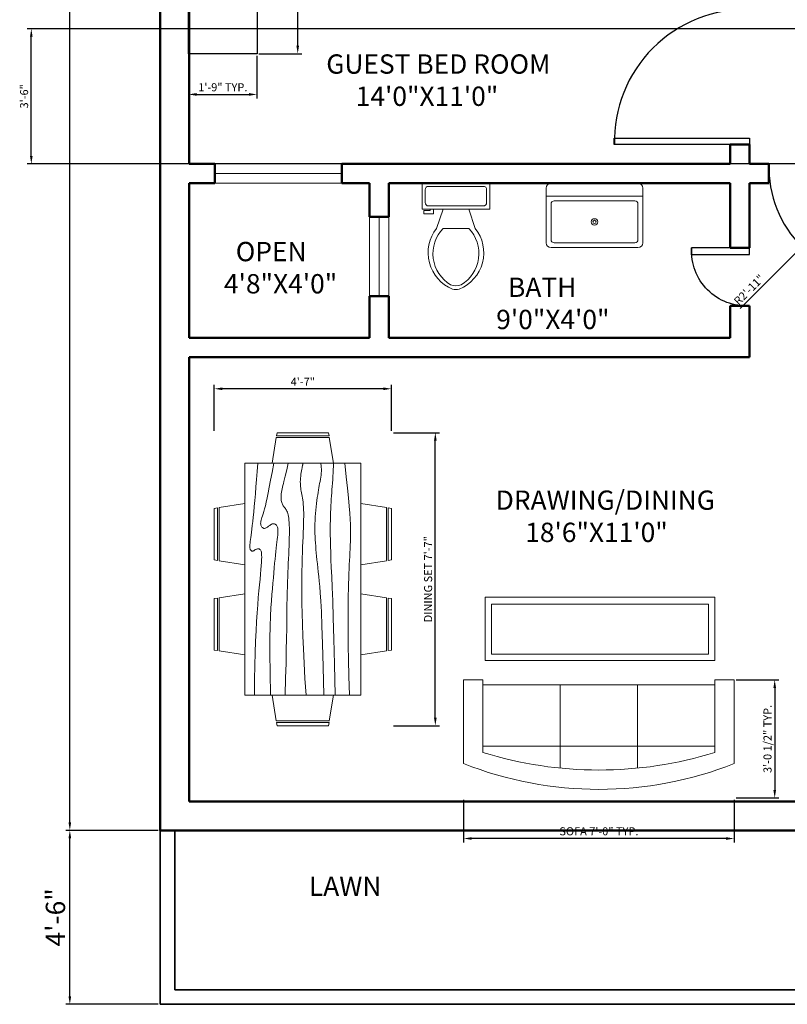
# Model space of a CAD drawing. Units: inches. Extents: x 2690 to 3266, y 1440 to 2261.
# Tile 1 of 4: x 2692 to 2930, y 1484 to 1790. Entities that reach past the tile are written whole.
import ezdxf

# ---------------------------------------------------------------- set-up
doc = ezdxf.new("R2010")
doc.units = ezdxf.units.IN
for name, color, linetype, lineweight in [('A-ANNO-DIMS', 2, 'Continuous', 18), ('A-AREA-IDEN', 7, 'Continuous', 25), ('A-DOOR', 4, 'Continuous', 25), ('A-FLOR-CASE', 9, 'Continuous', 25), ('A-FLOR-FIXT', 9, 'Continuous', 18), ('A-FURN', 8, 'Continuous', 18), ('A-GLAZ', 3, 'Continuous', 18), ('A-WALL', 7, 'Continuous', 50), ('L-SITE-WALL', 7, 'Continuous', 35)]:
    doc.layers.add(name, color=color, linetype=linetype, lineweight=lineweight)
doc.styles.get("Standard").update_dxf_attribs({"font": 'arial.ttf'})
doc.dimstyles.new('ISO-25', dxfattribs={"dimtxt": 2.5, "dimasz": 2.5, "dimexe": 1.25, "dimexo": 0.625, "dimtad": 1, "dimlunit": 3, "dimtxsty": 'Standard', "dimcen": 2.5, "dimadec": 0, "dimazin": 0, "dimtfac": 1, "dimtmove": 0, "dimatfit": 3, "dimfxl": 1, "dimarcsym": 0})

# ---------------------------------------------------------------- blocks, each defined once
blk = doc.blocks.new('Sofa - Roundback 7 ft.')
for p, q in [((-12.00002, -32.4421), (-12.00003, -6.5971)), ((11.99997, -32.4421), (11.99998, -6.5971)), ((-36.000027, -34), (-36.000027, -11.4696)), ((35.99998, -34), (35.99998, -11.4696)), ((-35.999844, -13.3819), (35.9998, -13.3819)), ((-36.000027, -32.4421), (35.99998, -32.4421))]:
    blk.add_line(p, q)
for points in [[(-36.000027, -34), (-42.000027, -34), (-42.000027, -8)], [(41.99998, -8), (41.99998, -34), (35.99998, -34)]]:
    blk.add_lwpolyline(points)
for centre, radius, start, end in [((0, -114.25), 114.25, 68.43141, 111.5686), ((-0.00001, -127.1968), 121.1968, 72.72033, 107.2797)]:
    blk.add_arc(centre, radius, start, end)
blk = doc.blocks.new('Dining Set - 36 x 72 in.')
for p, q in [((-22.2343, 26.00059), (-23.4847, 17.99762)), ((-22.2304, 26), (-5.7608, 26)), ((-22, 27.5), (-22.1562, 26.50042)), ((-5.8416, 26.5), (-22.1534, 26.5)), ((-22, 27.5), (-6, 27.5)), ((-5.8437, 26.49966), (-6, 27.5)), ((-4.5152, 17.99762), (-5.7655, 25.99926)), ((5.7657, 26.00059), (4.5153, 17.99762)), ((5.7696, 26), (22.2392, 26)), ((6, 27.5), (5.8438, 26.50042)), ((22.1584, 26.5), (5.8466, 26.5)), ((6, 27.5), (22, 27.5)), ((22.1563, 26.49966), (22, 27.5)), ((23.4848, 17.99762), (22.2345, 25.99926)), ((36, 18), (-36, 18)), ((-36, 18), (-36, -18)), ((36, -18), (36, 18)), ((-44.0006, 8.23428), (-35.9976, 9.48474)), ((44.0006, 8.23428), (35.9976, 9.48474)), ((-45.5, 8), (-44.5004, 8.15617)), ((-45.5, 8), (-45.5, -8)), ((-44.5, -8.15843), (-44.5, 8.15338)), ((-44, 8.23041), (-44, -8.23915)), ((44, 8.23041), (44, -8.23915)), ((44.5, -8.15843), (44.5, 8.15338)), ((45.5, 8), (44.5005, 8.15617)), ((45.5, 8), (45.5, -8)), ((-44.4997, -8.15631), (-45.5, -8)), ((-35.9976, -9.48476), (-43.9993, -8.2345)), ((35.9976, -9.48476), (43.9993, -8.2345)), ((44.4997, -8.15631), (45.5, -8)), ((-36, -18), (36, -18)), ((-22.2343, -26.0006), (-23.4847, -17.99762)), ((-4.5152, -17.99762), (-5.7655, -25.99928)), ((5.7657, -26.0006), (4.5153, -17.99762)), ((23.4848, -17.99762), (22.2345, -25.99928)), ((-22.2304, -26), (-5.7608, -26)), ((-22, -27.5), (-22.1562, -26.50044)), ((-5.8416, -26.5), (-22.1534, -26.5)), ((-22, -27.5), (-6, -27.5)), ((-5.8437, -26.49967), (-6, -27.5)), ((5.7696, -26), (22.2392, -26)), ((6, -27.5), (5.8438, -26.50044)), ((22.1584, -26.5), (5.8466, -26.5)), ((6, -27.5), (22, -27.5)), ((22.1563, -26.49967), (22, -27.5))]:
    blk.add_line(p, q)
for points in [[(-36, 15), (-31.1772, 14.97754), (-26.8079, 14.91406), (-22.8538, 14.81543), (-19.276, 14.6875), (-16.0362, 14.53613), (-13.0957, 14.36718), (-10.4159, 14.18652), (-7.9583, 14), (-5.6904, 13.81315), (-3.6035, 13.63021), (-1.6954, 13.45508), (0.0365, 13.29166), (1.5945, 13.14388), (2.9811, 13.01562), (4.1988, 12.9108), (5.25, 12.83333), (6.1393, 12.78613), (6.8802, 12.76823), (7.4883, 12.77767), (7.9792, 12.8125), (8.3685, 12.87077), (8.6719, 12.95052), (8.9049, 13.0498), (9.0833, 13.16666), (9.2205, 13.29899), (9.3216, 13.44401), (9.3895, 13.59879), (9.4271, 13.76041), (9.4373, 13.92594), (9.4232, 14.09245), (9.3875, 14.257), (9.3333, 14.41666), (9.2638, 14.56917), (9.1836, 14.71484), (9.0975, 14.85465), (9.0104, 14.98958), (8.9272, 15.1206), (8.8529, 15.2487), (8.7922, 15.37483), (8.75, 15.5), (8.7305, 15.62467), (8.7344, 15.74739), (8.7617, 15.86621), (8.8125, 15.97916), (8.8867, 16.08431), (8.9844, 16.17968), (9.1055, 16.26334), (9.25, 16.33333), (9.4189, 16.38802), (9.6172, 16.42708), (9.8506, 16.45052), (10.125, 16.45833), (10.4463, 16.45052), (10.8203, 16.42708), (11.2529, 16.38802), (11.75, 16.33333), (12.3184, 16.26318), (12.9694, 16.17838), (13.7151, 16.07991), (14.5677, 15.96875), (15.5395, 15.84586), (16.6426, 15.71224), (17.8893, 15.56884), (19.2917, 15.41666), (20.859, 15.25667), (22.5879, 15.08984), (24.4721, 14.91715), (26.5052, 14.73958), (28.6809, 14.5581), (30.9929, 14.3737), (33.4347, 14.18733), (36, 14)], [(-36, 10), (-28.9766, 10.14274), (-23.1725, 10.20442), (-18.4241, 10.19775), (-14.5677, 10.13541), (-11.4399, 10.03011), (-8.877, 9.89453), (-6.7154, 9.74137), (-4.7917, 9.58333), (-2.9698, 9.43082), (-1.2246, 9.28515), (0.4415, 9.14534), (2.026, 9.01041), (3.5266, 8.87939), (4.9408, 8.7513), (6.266, 8.62516), (7.5, 8.5), (8.6411, 8.37549), (9.6914, 8.2539), (10.6538, 8.13818), (11.5312, 8.03125), (12.3267, 7.93603), (13.043, 7.85547), (13.6831, 7.79248), (14.25, 7.75), (14.7471, 7.7303), (15.1797, 7.73307), (15.5537, 7.75732), (15.875, 7.80208), (16.1494, 7.86637), (16.3828, 7.94922), (16.5811, 8.04964), (16.75, 8.16666), (16.8944, 8.29915), (17.0143, 8.44531), (17.1089, 8.60319), (17.1771, 8.77083), (17.218, 8.94629), (17.2305, 9.1276), (17.2137, 9.31282), (17.1667, 9.5), (17.0895, 9.6875), (16.987, 9.875), (16.8649, 10.0625), (16.7292, 10.25), (16.5856, 10.4375), (16.4401, 10.625), (16.2985, 10.8125), (16.1667, 11), (16.05, 11.18733), (15.9518, 11.3737), (15.8752, 11.5581), (15.8229, 11.73958), (15.798, 11.91715), (15.8034, 12.08984), (15.842, 12.25667), (15.9167, 12.41666), (16.0295, 12.56836), (16.1784, 12.70833), (16.3605, 12.83268), (16.5729, 12.9375), (16.8127, 13.01888), (17.0768, 13.07291), (17.3625, 13.0957), (17.6667, 13.08333), (17.9894, 13.03312), (18.3418, 12.94726), (18.7382, 12.82918), (19.1927, 12.68229), (19.7195, 12.51001), (20.3327, 12.31575), (21.0465, 12.10294), (21.875, 11.875), (22.8357, 11.63354), (23.959, 11.37304), (25.2786, 11.08618), (26.8282, 10.76562), (28.6414, 10.40405), (30.752, 9.99414), (33.1936, 9.52856), (36, 9)], [(-36, 5.5), (-30.7157, 5.3348), (-26.069, 5.20963), (-21.9946, 5.11767), (-18.4271, 5.05208), (-15.3009, 5.00602), (-12.5508, 4.97265), (-10.1112, 4.94515), (-7.9167, 4.91666), (-5.909, 4.88167), (-4.0586, 4.83984), (-2.3429, 4.79215), (-0.7396, 4.73958), (0.7739, 4.6831), (2.22, 4.6237), (3.6213, 4.56233), (5, 4.5), (6.373, 4.43782), (7.7344, 4.3776), (9.0723, 4.32129), (10.375, 4.27083), (11.6309, 4.22819), (12.8281, 4.19531), (13.9551, 4.17415), (15, 4.16666), (15.954, 4.17448), (16.819, 4.19791), (17.6001, 4.23698), (18.3021, 4.29166), (18.9299, 4.36198), (19.4883, 4.44791), (19.9823, 4.54948), (20.4167, 4.66666), (20.7969, 4.79899), (21.1302, 4.94401), (21.4245, 5.09879), (21.6875, 5.26041), (21.9271, 5.42594), (22.1511, 5.59245), (22.3672, 5.757), (22.5834, 5.91666), (22.8065, 6.06868), (23.0404, 6.21093), (23.2879, 6.34147), (23.5521, 6.45833), (23.8358, 6.55957), (24.142, 6.64323), (24.4735, 6.70735), (24.8334, 6.75), (25.2235, 6.76969), (25.642, 6.76692), (26.0858, 6.74267), (26.5521, 6.69791), (27.0379, 6.63362), (27.5404, 6.55078), (28.0565, 6.45036), (28.5834, 6.33333), (29.1242, 6.19987), (29.7071, 6.04687), (30.3661, 5.87044), (31.1354, 5.66666), (32.0493, 5.43164), (33.142, 5.16146), (34.4475, 4.85221), (36, 4.5)], [(-36, -1), (-30.7915, -0.6591), (-26.0195, -0.38216), (-21.6519, -0.16284), (-17.6563, 0.00521), (-14.0005, 0.12833), (-10.6523, 0.21289), (-7.5796, 0.26522), (-4.75, 0.29166), (-2.134, 0.29793), (0.2878, 0.28711), (2.5317, 0.26163), (4.6146, 0.22396), (6.5529, 0.17651), (8.3633, 0.12174), (10.0623, 0.06209), (11.6667, 0), (13.1899, -0.06201), (14.6341, -0.1211), (15.9982, -0.17432), (17.2813, -0.21875), (18.4823, -0.25147), (19.6003, -0.26953), (20.6343, -0.27002), (21.5834, -0.25), (22.4481, -0.20768), (23.2357, -0.14584), (23.9549, -0.06836), (24.6146, 0.02083), (25.2235, 0.11784), (25.7904, 0.21875), (26.3241, 0.31966), (26.8334, 0.41666), (27.3265, 0.50618), (27.8099, 0.58593), (28.2894, 0.65397), (28.7709, 0.70833), (29.2601, 0.74707), (29.763, 0.76823), (30.2855, 0.76985), (30.8334, 0.75), (31.4088, 0.70784), (31.9994, 0.64713), (32.589, 0.57275), (33.1615, 0.48958), (33.7008, 0.4025), (34.1908, 0.3164), (34.6153, 0.23616), (34.9584, 0.16666), (35.2099, 0.11165), (35.3848, 0.07031), (35.504, 0.04069), (35.5886, 0.02083), (35.6594, 0.00879), (35.7377, 0.0026), (35.8442, 0.00032), (36, 0)], [(-36, -6.5), (-27.1843, -6.31267), (-20.084, -6.1263), (-14.469, -5.9419), (-10.1094, -5.76042), (-6.7752, -5.58285), (-4.2363, -5.41016), (-2.2629, -5.24333), (-0.625, -5.08334), (0.8708, -4.93099), (2.2715, -4.78646), (3.5872, -4.64974), (4.8281, -4.52084), (6.0046, -4.39974), (7.127, -4.28646), (8.2053, -4.18099), (9.25, -4.08334), (10.2705, -3.99382), (11.2734, -3.91407), (12.2647, -3.84603), (13.25, -3.79167), (14.2354, -3.75293), (15.2266, -3.73177), (16.2295, -3.73015), (17.25, -3.75), (18.2912, -3.79248), (19.3451, -3.85547), (20.4009, -3.93604), (21.4479, -4.03125), (22.4754, -4.13819), (23.4727, -4.25391), (24.4289, -4.37549), (25.3334, -4.5), (26.1785, -4.62492), (26.9694, -4.74935), (27.7145, -4.87281), (28.4219, -4.99479), (29.1, -5.11483), (29.7572, -5.23242), (30.4016, -5.34709), (31.0417, -5.45834), (31.6837, -5.56437), (32.3262, -5.65821), (32.9658, -5.73153), (33.599, -5.77604), (34.2224, -5.78345), (34.8327, -5.74545), (35.4264, -5.65373), (36, -5.5)], [(-36, -10), (-26.4022, -9.81299), (-18.4675, -9.62891), (-11.9839, -9.45069), (-6.7396, -9.28125), (-2.5226, -9.12354), (0.8789, -8.98047), (3.6769, -8.85498), (6.0833, -8.75), (8.2767, -8.66765), (10.3021, -8.60677), (12.1712, -8.56543), (13.8958, -8.54167), (15.4876, -8.53353), (16.9583, -8.53907), (18.3197, -8.55632), (19.5834, -8.58334), (20.7616, -8.61841), (21.8685, -8.66081), (22.9188, -8.71004), (23.9271, -8.76563), (24.9081, -8.82707), (25.8763, -8.89388), (26.8465, -8.96558), (27.8334, -9.04167), (28.8474, -9.12118), (29.8828, -9.20117), (30.93, -9.27824), (31.9792, -9.34896), (33.0205, -9.40991), (34.0443, -9.45768), (35.0407, -9.48885), (36, -9.5)], [(-36, -14.5), (-30.0881, -14.33513), (-25.0332, -14.21224), (-20.7312, -14.12647), (-17.0781, -14.07292), (-13.97, -14.04671), (-11.3027, -14.04297), (-8.9724, -14.05681), (-6.875, -14.08334), (-4.9224, -14.11833), (-3.0905, -14.16016), (-1.3709, -14.20785), (0.2448, -14.26042), (1.7647, -14.3169), (3.1973, -14.3763), (4.5507, -14.43767), (5.8333, -14.5), (7.0554, -14.5621), (8.235, -14.62175), (9.3922, -14.67652), (10.5469, -14.72396), (11.7192, -14.76164), (12.929, -14.78711), (14.1965, -14.79794), (15.5417, -14.79167), (16.9933, -14.76424), (18.6152, -14.70508), (20.4804, -14.60197), (22.6615, -14.44271), (25.2312, -14.21509), (28.2624, -13.9069), (31.8277, -13.50594), (36, -13)]]:
    blk.add_lwpolyline(points)
blk = doc.blocks.new('Toilet - top')
for p, q in [((9.5, -6), (9.5, -2)), ((-10, -8.5), (-8, -8.5)), ((-10, -9.5), (-10, -8.5)), ((-8, -8.5), (-8, -8)), ((-7, -8), (-7, -9.5)), ((-4, -8), (-6, -14)), ((4, -8), (6, -14)), ((-7, -9.5), (-10, -9.5)), ((4, -14), (-4, -14))]:
    blk.add_line(p, q)
blk.add_lwpolyline([(10.5, -8), (10.5, 0), (-10.5, 0), (-10.5, -8)], close=True)
for points in [[(-9.5, -2), (-9.5, -6)], [(8.5, -1), (-8.5, -1)], [(-8.5, -7), (8.5, -7)]]:
    blk.add_lwpolyline(points)
for centre, radius, start, end in [((-8.62, -1.88), 0.884, 81.8699, 188.1301), ((8.62, -1.88), 0.884, 351.8699, 98.1301), ((-8.62, -6.12), 0.884, 171.8699, 278.1301), ((8.62, -6.12), 0.884, 261.8699, 8.1301), ((3.52, -21.58), 12.17, 141.4691, 247.9714), ((4.2, -21.82), 11.33, 136.3677, 238.9468), ((-3.52, -21.58), 12.17, 292.0284, 38.5307), ((-4.2, -21.82), 11.33, 301.053, 43.6321), ((0, -27.88), 4, 245.7318, 294.2682), ((0, -29), 4, 254.8605, 285.1395)]:
    blk.add_arc(centre, radius, start, end)
blk = doc.blocks.new('Sink-single - 30 in top')
blk.add_line((-15, -3.999996), (15, -3.999996))
for points in [[(-13.5, 0), (13.5, 0)], [(-15, -18.499996), (-15, -1.5)], [(15, -1.5), (15, -18.499996)], [(-12.5, -5.499996), (12.5, -5.499996)], [(-13.5, -17.499996), (-13.5, -6.499996)], [(13.5, -6.499996), (13.5, -17.499996)], [(13.5, -19.999996), (-13.5, -19.999996)], [(12.5, -18.499996), (-12.5, -18.499996)]]:
    blk.add_lwpolyline(points)
for radius in [1, 0.5]:
    blk.add_circle((0, -11.999996), radius)
for centre, radius, start, end in [((-13.5, -1.5), 1.5, 90, 180), ((13.5, -1.5), 1.5, 0, 90), ((-12.5, -6.499996), 1, 90, 180), ((12.5, -6.499996), 1, 0, 90), ((-12.5, -17.499996), 1, 180, 270), ((12.5, -17.499996), 1, 270, 0), ((-13.5, -18.499996), 1.5, 180, 270), ((13.5, -18.499996), 1.5, 270, 0)]:
    blk.add_arc(centre, radius, start, end)
blk = doc.blocks.new('*D13')
at = {"layer": 'A-ANNO-DIMS', "color": 0, "lineweight": -2, "transparency": 16777216}
for p, q in [((2734.85, 2204.49), (2706.14, 2204.49)), ((2707.39, 1540.99), (2707.39, 2201.99)), ((2734.85, 1538.49), (2706.14, 1538.49))]:
    blk.add_line(p, q, dxfattribs=at)
at = {"layer": 'A-ANNO-DIMS', "color": 0, "transparency": 16777216}
for points in [[(2706.97, 2201.99), (2707.81, 2201.99), (2707.39, 2204.49)], [(2706.97, 1540.99), (2707.81, 1540.99), (2707.39, 1538.49)]]:
    blk.add_solid(points, dxfattribs=at)
at = {"layer": 'Defpoints', "color": 0, "transparency": 16777216}
for p in [(2707.39, 2204.49), (2735.48, 2204.49), (2735.48, 1538.49)]:
    blk.add_point(p, dxfattribs=at)
at = {"layer": 'A-ANNO-DIMS', "color": 0, "transparency": 16777216, "insert": (2703.7, 1871.49), "char_height": 6, "attachment_point": 5, "rotation": 90}
blk.add_mtext('55\'-6"', dxfattribs=at)
blk = doc.blocks.new('*D14')
at = {"layer": 'A-ANNO-DIMS', "color": 0, "lineweight": -2, "transparency": 16777216}
for p, q in [((2734.85, 1538.49), (2706.14, 1538.49)), ((2707.39, 1486.99), (2707.39, 1535.99)), ((2734.85, 1484.49), (2706.14, 1484.49))]:
    blk.add_line(p, q, dxfattribs=at)
at = {"layer": 'A-ANNO-DIMS', "color": 0, "transparency": 16777216}
for points in [[(2706.97, 1535.99), (2707.81, 1535.99), (2707.39, 1538.49)], [(2706.97, 1486.99), (2707.81, 1486.99), (2707.39, 1484.49)]]:
    blk.add_solid(points, dxfattribs=at)
at = {"layer": 'Defpoints', "color": 0, "transparency": 16777216}
for p in [(2707.39, 1538.49), (2735.48, 1538.49), (2735.48, 1484.49)]:
    blk.add_point(p, dxfattribs=at)
at = {"layer": 'A-ANNO-DIMS', "color": 0, "transparency": 16777216, "insert": (2703.7, 1511.49), "char_height": 6, "attachment_point": 5, "rotation": 90}
blk.add_mtext('4\'-6"', dxfattribs=at)
blk = doc.blocks.new('DOOR-SWING-18IN')
for p, q in [((0, 0), (0, 18)), ((0, 18), (2, 18)), ((2, 18), (2, 0)), ((2, 0), (0, 0))]:
    blk.add_line(p, q)
blk.add_arc((1, 1), 17.03, 356.6335, 93.3665)
blk = doc.blocks.new('DOOR-SWING-42IN')
for p, q in [((-42, 0), (-42, 2)), ((-42, 2), (0, 2)), ((0, 0), (-42, 0)), ((0, 2), (0, 0))]:
    blk.add_line(p, q)
blk.add_arc((-1, 1), 41.01, 88.6028, 181.3972)
blk = doc.blocks.new('WARDROBE-PLAN')
blk.add_lwpolyline([(0, 0), (21.23, 0), (21.23, -84.36), (0, -84.36)], close=True)
blk = doc.blocks.new('*D31')
at = {"layer": 'A-ANNO-DIMS', "color": 0, "lineweight": -2, "transparency": 16777216}
for p, q in [((2766.13, 1864.09), (2779.41, 1864.09)), ((2778.16, 1782.23), (2778.16, 1861.59)), ((2766.13, 1779.73), (2779.41, 1779.73))]:
    blk.add_line(p, q, dxfattribs=at)
at = {"layer": 'A-ANNO-DIMS', "color": 0, "transparency": 16777216}
for points in [[(2777.74, 1861.59), (2778.58, 1861.59), (2778.16, 1864.09)], [(2777.74, 1782.23), (2778.58, 1782.23), (2778.16, 1779.73)]]:
    blk.add_solid(points, dxfattribs=at)
at = {"layer": 'Defpoints', "color": 0, "transparency": 16777216}
for p in [(2765.51, 1864.09), (2778.16, 1864.09), (2765.51, 1779.73)]:
    blk.add_point(p, dxfattribs=at)
at = {"layer": 'A-ANNO-DIMS', "color": 0, "transparency": 16777216, "insert": (2776.24, 1821.91), "char_height": 2.5, "attachment_point": 5, "rotation": 90}
blk.add_mtext('WARDROBE 7\'-0 1/2" TYP.', dxfattribs=at)
blk = doc.blocks.new('*D32')
at = {"layer": 'A-ANNO-DIMS', "color": 0, "lineweight": -2, "transparency": 16777216}
for p, q in [((2744.28, 1779.11), (2744.28, 1765.83)), ((2765.51, 1779.11), (2765.51, 1765.83)), ((2746.78, 1767.08), (2763.01, 1767.08))]:
    blk.add_line(p, q, dxfattribs=at)
at = {"layer": 'A-ANNO-DIMS', "color": 0, "transparency": 16777216}
for points in [[(2746.78, 1767.5), (2746.78, 1766.66), (2744.28, 1767.08)], [(2763.01, 1767.5), (2763.01, 1766.66), (2765.51, 1767.08)]]:
    blk.add_solid(points, dxfattribs=at)
at = {"layer": 'Defpoints', "color": 0, "transparency": 16777216}
for p in [(2744.28, 1779.73), (2765.51, 1779.73), (2765.51, 1767.08)]:
    blk.add_point(p, dxfattribs=at)
at = {"layer": 'A-ANNO-DIMS', "color": 0, "transparency": 16777216, "insert": (2754.9, 1768.98), "char_height": 2.5, "attachment_point": 5}
blk.add_mtext('1\'-9" TYP.', dxfattribs=at)
blk = doc.blocks.new('*D33')
at = {"layer": 'A-ANNO-DIMS', "color": 0, "lineweight": -2, "transparency": 16777216}
for p, q in [((2829.68, 1547.95), (2829.68, 1534.73)), ((2913.68, 1547.95), (2913.68, 1534.73)), ((2911.18, 1535.98), (2832.18, 1535.98))]:
    blk.add_line(p, q, dxfattribs=at)
at = {"layer": 'A-ANNO-DIMS', "color": 0, "transparency": 16777216}
for points in [[(2832.18, 1536.4), (2832.18, 1535.56), (2829.68, 1535.98)], [(2911.18, 1536.4), (2911.18, 1535.56), (2913.68, 1535.98)]]:
    blk.add_solid(points, dxfattribs=at)
at = {"layer": 'Defpoints', "color": 0, "transparency": 16777216}
for p in [(2829.68, 1548.58), (2913.68, 1548.58), (2829.68, 1535.98)]:
    blk.add_point(p, dxfattribs=at)
at = {"layer": 'A-ANNO-DIMS', "color": 0, "transparency": 16777216, "insert": (2871.68, 1537.9), "char_height": 2.5, "attachment_point": 5}
blk.add_mtext('SOFA 7\'-0" TYP.', dxfattribs=at)
blk = doc.blocks.new('*D34')
at = {"layer": 'A-ANNO-DIMS', "color": 0, "lineweight": -2, "transparency": 16777216}
for p, q in [((2914.31, 1585.25), (2927.53, 1585.25)), ((2926.28, 1582.75), (2926.28, 1551.08)), ((2914.31, 1548.58), (2927.53, 1548.58))]:
    blk.add_line(p, q, dxfattribs=at)
at = {"layer": 'A-ANNO-DIMS', "color": 0, "transparency": 16777216}
for points in [[(2925.87, 1582.75), (2926.7, 1582.75), (2926.28, 1585.25)], [(2925.87, 1551.08), (2926.7, 1551.08), (2926.28, 1548.58)]]:
    blk.add_solid(points, dxfattribs=at)
at = {"layer": 'Defpoints', "color": 0, "transparency": 16777216}
for p in [(2913.68, 1585.25), (2913.68, 1548.58), (2926.28, 1548.58)]:
    blk.add_point(p, dxfattribs=at)
at = {"layer": 'A-ANNO-DIMS', "color": 0, "transparency": 16777216, "insert": (2924.37, 1566.91), "char_height": 2.5, "attachment_point": 5, "rotation": 90}
blk.add_mtext('3\'-0 1/2" TYP.', dxfattribs=at)
blk = doc.blocks.new('*D41')
at = {"layer": 'A-ANNO-DIMS', "color": 0, "lineweight": -2, "transparency": 16777216}
for p, q in [((2807.86, 1662.01), (2822.14, 1662.01)), ((2820.89, 1573.51), (2820.89, 1659.51)), ((2807.86, 1571.01), (2822.14, 1571.01))]:
    blk.add_line(p, q, dxfattribs=at)
at = {"layer": 'A-ANNO-DIMS', "color": 0, "transparency": 16777216}
for points in [[(2820.47, 1659.51), (2821.31, 1659.51), (2820.89, 1662.01)], [(2820.47, 1573.51), (2821.31, 1573.51), (2820.89, 1571.01)]]:
    blk.add_solid(points, dxfattribs=at)
at = {"layer": 'Defpoints', "color": 0, "transparency": 16777216}
for p in [(2807.24, 1662.01), (2820.89, 1662.01), (2807.24, 1571.01)]:
    blk.add_point(p, dxfattribs=at)
at = {"layer": 'A-ANNO-DIMS', "color": 0, "transparency": 16777216, "insert": (2818.97, 1616.51), "char_height": 2.5, "attachment_point": 5, "rotation": 90}
blk.add_mtext('DINING SET 7\'-7"', dxfattribs=at)
blk = doc.blocks.new('*D42')
at = {"layer": 'A-ANNO-DIMS', "color": 0, "lineweight": -2, "transparency": 16777216}
for p, q in [((2752.24, 1662.63), (2752.24, 1676.91)), ((2807.24, 1662.63), (2807.24, 1676.91)), ((2804.74, 1675.66), (2754.74, 1675.66))]:
    blk.add_line(p, q, dxfattribs=at)
at = {"layer": 'A-ANNO-DIMS', "color": 0, "transparency": 16777216}
for points in [[(2754.74, 1676.07), (2754.74, 1675.24), (2752.24, 1675.66)], [(2804.74, 1676.07), (2804.74, 1675.24), (2807.24, 1675.66)]]:
    blk.add_solid(points, dxfattribs=at)
at = {"layer": 'Defpoints', "color": 0, "transparency": 16777216}
for p in [(2752.24, 1675.66), (2752.24, 1662.01), (2807.24, 1662.01)]:
    blk.add_point(p, dxfattribs=at)
at = {"layer": 'A-ANNO-DIMS', "color": 0, "transparency": 16777216, "insert": (2779.74, 1677.53), "char_height": 2.5, "attachment_point": 5}
blk.add_mtext('4\'-7"', dxfattribs=at)
blk = doc.blocks.new('*D53')
at = {"layer": 'A-ANNO-DIMS', "color": 0, "lineweight": -2, "transparency": 16777216}
for p, q in [((3073.85, 1787.49), (2694.18, 1787.49)), ((2695.43, 1747.99), (2695.43, 1784.99)), ((3073.85, 1745.49), (2694.18, 1745.49))]:
    blk.add_line(p, q, dxfattribs=at)
at = {"layer": 'A-ANNO-DIMS', "color": 0, "transparency": 16777216}
for points in [[(2695.01, 1784.99), (2695.84, 1784.99), (2695.43, 1787.49)], [(2695.01, 1747.99), (2695.84, 1747.99), (2695.43, 1745.49)]]:
    blk.add_solid(points, dxfattribs=at)
at = {"layer": 'Defpoints', "color": 0, "transparency": 16777216}
for p in [(2695.43, 1787.49), (3074.48, 1787.49), (3074.48, 1745.49)]:
    blk.add_point(p, dxfattribs=at)
at = {"layer": 'A-ANNO-DIMS', "color": 0, "transparency": 16777216, "insert": (2693.52, 1766.49), "char_height": 2.5, "attachment_point": 5, "rotation": 90}
blk.add_mtext('3\'-6"', dxfattribs=at)
blk = doc.blocks.new('*D61')
at = {"layer": 'A-ANNO-DIMS', "color": 0, "lineweight": -2, "transparency": 16777216}
for p, q in [((2959.48, 1744.49), (2934.72, 1719.73)), ((2915.54, 1700.55), (2932.95, 1717.96))]:
    blk.add_line(p, q, dxfattribs=at)
at = {"layer": 'A-ANNO-DIMS', "color": 0, "transparency": 16777216}
blk.add_solid([(2932.65, 1718.25), (2933.24, 1717.66), (2934.72, 1719.73)], dxfattribs=at)
at = {"layer": 'Defpoints', "color": 0, "transparency": 16777216}
for p in [(2959.48, 1744.49), (2934.72, 1719.73)]:
    blk.add_point(p, dxfattribs=at)
at = {"layer": 'A-ANNO-DIMS', "color": 0, "transparency": 16777216, "insert": (2918.53, 1706.2), "char_height": 2.5, "attachment_point": 5, "rotation": 44.9992}
blk.add_mtext('R2\'-11"', dxfattribs=at)

msp = doc.modelspace()

# ---------------------------------------------------------------- linework, layer by layer
at = {"layer": 'A-DOOR'}
msp.add_line((2918.476, 1751.486), (2918.476, 1751.486), dxfattribs=at)
msp.add_arc((2959.476, 1744.486), 35.014, 178.36342, 271.63658, dxfattribs=at)
at = {"layer": 'A-FURN'}
for points in [[(2836.32, 1610.936), (2907.685, 1610.936), (2907.685, 1591.299), (2836.32, 1591.299)], [(2838.284, 1608.799), (2905.73, 1608.799), (2905.73, 1593.248), (2838.284, 1593.248)]]:
    msp.add_lwpolyline(points, close=True, dxfattribs=at)
at = {"layer": 'A-GLAZ'}
for p, q in [((2752.427, 1745.486), (2791.813, 1745.486)), ((2791.813, 1745.486), (2791.813, 1742.486)), ((2791.813, 1742.486), (2752.427, 1742.486)), ((2752.427, 1742.486), (2752.427, 1739.486)), ((2752.427, 1739.486), (2791.813, 1739.486)), ((2800.476, 1729.052), (2800.476, 1704.39)), ((2803.476, 1704.39), (2803.476, 1729.052)), ((2803.476, 1729.052), (2806.476, 1729.052)), ((2806.476, 1729.052), (2806.476, 1704.39)), ((2800.476, 1704.39), (2803.476, 1704.39))]:
    msp.add_line(p, q, dxfattribs=at)
at = {"layer": 'A-WALL'}
for p, q in [((2735.476, 1538.486), (2735.476, 2204.486)), ((2744.476, 1745.486), (2744.476, 1877.486)), ((2912.476, 1745.486), (2912.476, 1751.486)), ((2918.476, 1751.486), (2912.476, 1751.486)), ((2918.476, 1745.486), (2918.476, 1751.486)), ((2918.476, 1745.486), (2918.476, 1751.486)), ((2744.476, 1745.486), (2752.427, 1745.486)), ((2752.427, 1745.486), (2752.427, 1739.486)), ((2791.813, 1745.486), (2791.813, 1739.486)), ((2791.813, 1745.486), (2912.476, 1745.486)), ((2924.476, 1745.486), (2918.476, 1745.486)), ((2924.476, 1739.486), (2924.476, 1745.486)), ((2744.476, 1739.486), (2752.427, 1739.486)), ((2744.476, 1691.486), (2744.476, 1739.486)), ((2791.813, 1739.486), (2800.476, 1739.486)), ((2800.476, 1729.052), (2800.476, 1739.486)), ((2806.476, 1739.486), (2912.476, 1739.486)), ((2806.476, 1729.052), (2806.476, 1739.486)), ((2912.476, 1719.41), (2912.476, 1739.486)), ((2918.476, 1739.486), (2924.476, 1739.486)), ((2918.476, 1719.41), (2918.476, 1739.486)), ((2800.476, 1729.052), (2806.476, 1729.052)), ((2912.476, 1719.41), (2918.476, 1719.41)), ((2800.476, 1691.486), (2800.476, 1704.39)), ((2800.476, 1704.39), (2806.476, 1704.39)), ((2806.476, 1691.486), (2806.476, 1704.39)), ((2912.476, 1691.486), (2912.476, 1701.41)), ((2912.476, 1701.41), (2918.476, 1701.41)), ((2918.476, 1685.486), (2918.476, 1701.41)), ((2744.476, 1691.486), (2800.476, 1691.486)), ((2806.476, 1691.486), (2912.476, 1691.486)), ((2744.476, 1547.486), (2744.476, 1685.486)), ((2744.476, 1685.486), (2918.476, 1685.486)), ((2966.476, 1547.486), (2744.476, 1547.486)), ((2972.476, 1538.486), (2735.476, 1538.486))]:
    msp.add_line(p, q, dxfattribs=at)
at = {"layer": 'L-SITE-WALL'}
for p, q in [((2735.476, 1538.486), (2735.476, 1484.486)), ((2739.976, 1538.486), (2739.976, 1488.986)), ((2739.976, 1488.986), (2989.13, 1488.986)), ((2735.476, 1484.486), (2989.13, 1484.486))]:
    msp.add_line(p, q, dxfattribs=at)

# ---------------------------------------------------------------- block references
at = {"layer": 'A-DOOR'}
msp.add_blockref('DOOR-SWING-42IN', (2918.476, 1751.486), dxfattribs=at)
at = {"layer": 'A-DOOR', "extrusion": (0, 0, -1), "zscale": -1, "rotation": 270.000000000001}
msp.add_blockref('DOOR-SWING-18IN', (-2918.476, 1719.41), dxfattribs=at)
at = {"layer": 'A-FLOR-CASE'}
msp.add_blockref('WARDROBE-PLAN', (2744.283, 1864.093), dxfattribs=at)
at = {"layer": 'A-FLOR-FIXT'}
for name, p in [('Toilet - top', (2827.281, 1739.486)), ('Sink-single - 30 in top', (2870.327, 1739.486))]:
    msp.add_blockref(name, p, dxfattribs=at)
at = {"layer": 'A-FURN'}
for name, p, rotation in [('Dining Set - 36 x 72 in.', (2779.739, 1616.507), 90), ('Sofa - Roundback 7 ft.', (2871.685, 1551.245), 180)]:
    msp.add_blockref(name, p, dxfattribs=dict(at, rotation=rotation))

# ---------------------------------------------------------------- texts
at = {"layer": 'A-AREA-IDEN', "char_height": 6, "attachment_point": 1}
for s, width, heights, insert in [('     GUEST BED ROOM\\P          14\'0"X11\'0"', 101.41733, [40.167], (2777.848, 1779.519)), ('     OPEN\\P   4\'8"X4\'0"', 77.52183, [0], (2749.753, 1721.272)), ('  BATH\\P9\'0"X4\'0"', 77.52183, [0], (2839.799, 1710.186)), ('DRAWING/DINING\\P     18\'6"X11\'0"', 77.52183, [0], (2839.644, 1644.065)), ('   LAWN', 77.52183, [0], (2776.129, 1524.157))]:
    msp.add_mtext_dynamic_manual_height_columns(s, width=width, gutter_width=12.5, heights=heights, dxfattribs=dict(at, insert=insert))

# ---------------------------------------------------------------- dimensions: what is measured, and where the dimension line sits
at = {"layer": 'A-ANNO-DIMS'}
for base, p1, p2, angle, override, picture, middle in [((2707.39, 2204.486), (2735.476, 1538.486), (2735.476, 2204.486), 90, {"dimtxt": 6, "dimclrd": 0, "dimclre": 0, "dimclrt": 0}, '*D13', (2703.701, 1871.486)), ((2695.426, 1787.486), (3074.476, 1745.486), (3074.476, 1787.486), 90, {"dimdec": 1, "dimlfac": 1, "dimrnd": 0, "dimzin": 1, "dimdsep": 46, "dimlunit": 4, "dimfrac": 2}, '*D53', (2693.524, 1766.486)), ((2752.239, 1675.657), (2807.239, 1662.007), (2752.239, 1662.007), 180, {"dimdec": 1, "dimlfac": 1, "dimrnd": 0, "dimzin": 1, "dimdsep": 46, "dimlunit": 4, "dimfrac": 2}, '*D42', (2779.739, 1677.532)), ((2707.39, 1538.486), (2735.476, 1484.486), (2735.476, 1538.486), 90, {"dimtxt": 6, "dimclrd": 0, "dimclre": 0, "dimclrt": 0}, '*D14', (2703.701, 1511.486))]:
    dim = msp.add_linear_dim(base=base, p1=p1, p2=p2, angle=angle, dimstyle='ISO-25', override=override, dxfattribs=at)
    dim.commit()
    dim.dimension.update_dxf_attribs({"geometry": picture, "text_midpoint": middle})
for base, p1, p2, angle, text, picture, middle in [((2778.162, 1864.093), (2765.508, 1779.735), (2765.508, 1864.093), 90, 'WARDROBE <> TYP.', '*D31', (2776.243, 1821.914)), ((2820.889, 1662.007), (2807.239, 1571.007), (2807.239, 1662.007), 90, 'DINING SET <>', '*D41', (2818.971, 1616.507)), ((2926.285, 1548.579), (2913.685, 1585.245), (2913.685, 1548.579), 270, '<> TYP.', '*D34', (2924.366, 1566.912)), ((2829.685, 1535.979), (2913.685, 1548.579), (2829.685, 1548.579), 180, 'SOFA <> TYP.', '*D33', (2871.685, 1537.897))]:
    dim = msp.add_linear_dim(base=base, p1=p1, p2=p2, angle=angle, text=text, dimstyle='ISO-25', override={"dimdec": 1, "dimlfac": 1, "dimrnd": 0, "dimzin": 1, "dimdsep": 46, "dimlunit": 4, "dimfrac": 2}, dxfattribs=at)
    dim.commit()
    dim.dimension.update_dxf_attribs({"geometry": picture, "text_midpoint": middle})
dim = msp.add_linear_dim(base=(2765.508, 1767.081), p1=(2744.283, 1779.735), p2=(2765.508, 1779.735), text='<> TYP.', dimstyle='ISO-25', override={"dimdec": 1, "dimlfac": 1, "dimrnd": 0, "dimzin": 1, "dimdsep": 46, "dimlunit": 4, "dimfrac": 2}, dxfattribs=at)
dim.commit()
dim.dimension.update_dxf_attribs({"geometry": '*D32', "text_midpoint": (2754.895, 1768.982)})
dim = msp.add_radius_dim(center=(2959.476, 1744.486), mpoint=(2934.717, 1719.727), dimstyle='ISO-25', override={"dimdec": 1, "dimlfac": 1, "dimrnd": 0, "dimzin": 1, "dimdsep": 46, "dimlunit": 4, "dimfrac": 2}, dxfattribs=at)
dim.commit()
dim.dimension.update_dxf_attribs({"geometry": '*D61', "text_midpoint": (2919.862, 1704.872), "dimtype": 164})

doc.saveas('drawing.dxf')
